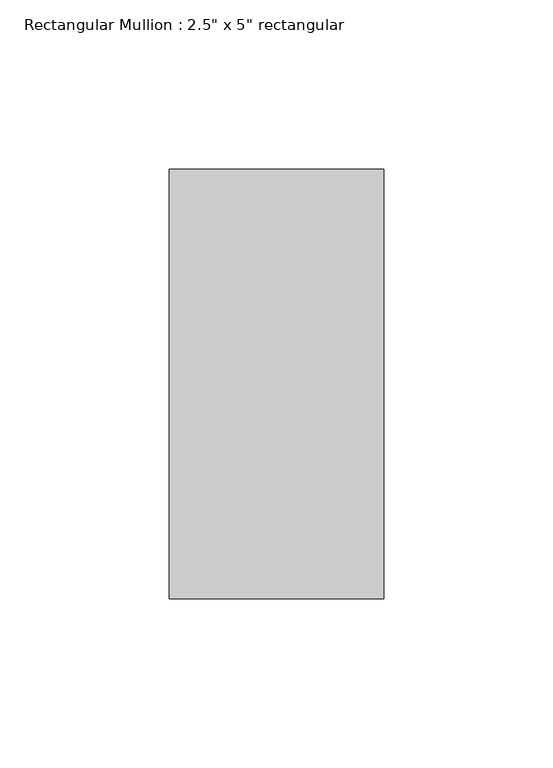
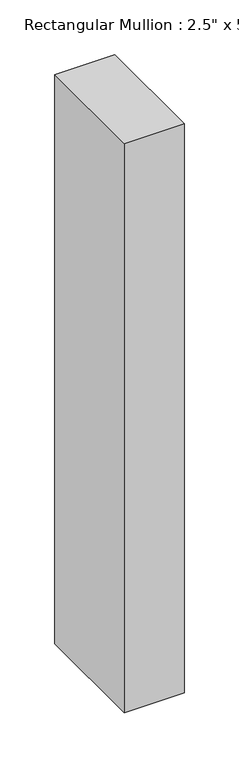
"""IFC4 building model written with IfcOpenShell, lengths in millimetres: member geometry."""

from ifc_helpers import new_model, si_unit, frame, origin, place, context, project, spatial, polyline, outline, extrude, source, transform, mapped, element, save


def member_06d1cbbd(model_context):
    return source(origin(), model_context, "Body", "SweptSolid", [
        extrude(outline(polyline([(0.0, 63.5), (0.0, -63.5), (-63.5, -63.5), (-63.5, 63.5), (0.0, 63.5)])), frame((0.0, 0.0, -636.2206626), z_axis=(0.0, 0.0, 1.0), x_axis=(1.0, 0.0, 0.0)), (0.0, 0.0, 1.0), 636.2206626),
    ])


if __name__ == "__main__":
    model = new_model("IFC4")
    model_context = context("Model", 3, world=origin())
    ifc_project = project(units=[si_unit("LENGTHUNIT", "METRE", prefix="MILLI")], contexts=[model_context])
    site = spatial("IfcSite", under=ifc_project)
    building = spatial("IfcBuilding", under=site)
    placement = place(None, origin())
    member_shape = member_06d1cbbd(model_context)
    element("IfcMember", 1, ObjectType="Rectangular Mullion : 2.5\" x 5\" rectangular", at=placement, inside=building, context=model_context, shape_type="MappedRepresentation", body=[
        mapped(member_shape, transform((0.0, 0.0, 0.0), x_axis=(1.0, 0.0, 0.0), y_axis=(0.0, 1.0, 0.0), z_axis=(0.0, 0.0, 1.0))),
    ])
    save(model, "model.ifc")

# Revit data of these elements
# Type "Rectangular Mullion : 2.5\" x 5\" rectangular"
#   built-in parameter 1007304 = 0.416667 (stored number, unit not read)
#   built-in parameter 1007301 = 0.104167 (stored number, unit not read)
#   built-in parameter 1007300 = 0.104167 (stored number, unit not read)
# Element 1 (IfcMember, "Rectangular Mullion : 2.5\" x 5\" rectangular")
#   Materials on its faces: "Aluminum"
# Materials
#   "Aluminum": class "Metal", colour RGB 247 247 247, transparency 0, Description = "Aluminum 6061", Cost = 0
